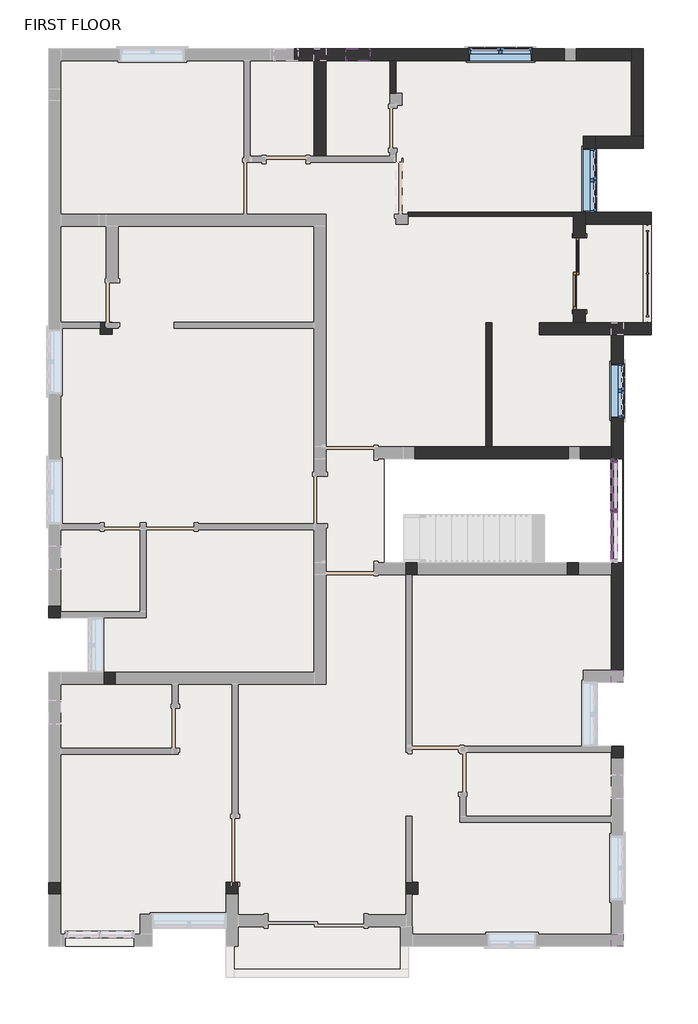
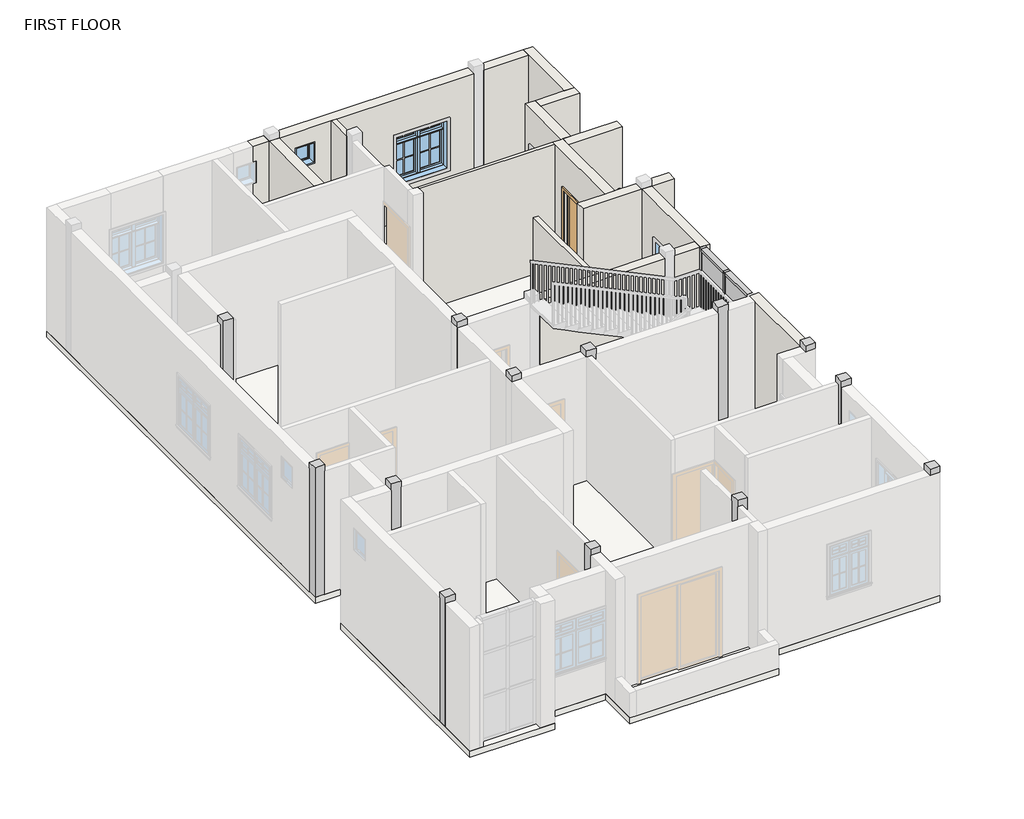
# One storey, part 3 of 6: 17 walls, 13 columns, 9 members, 4 plates, 4 windows, 1 door, 1 slab.
"""IFC4 building model written with IfcOpenShell, lengths in millimetres."""

from ifc_helpers import new_model, si_unit, frame, origin, place, context, project, spatial, polyline, outline, extrude, faceted_brep, transform, mapped, element, save
from components import door_double_sliding_4_5_x7_60868813, member_f1f71bde, member_e0487b50, member_aafbdc53, member_00c01c4d, member_0131f3aa, member_ecafcbb3, system_panel_glazed_149319f3, system_panel_glazed_118543cb, window_abb441dd, window_35f3c129, window_casement_double_awning_double_4_x4_dd9041c6

model = new_model("IFC4")

# Units and contexts
model_context = context("Model", 3, world=origin())
ifc_project = project(units=[si_unit("LENGTHUNIT", "METRE", prefix="MILLI")], contexts=[model_context])

# Site, building, storey
site = spatial("IfcSite", under=ifc_project)
building = spatial("IfcBuilding", under=site)
storey = spatial("IfcBuildingStorey", under=building, Name="FIRST FLOOR", Elevation=3200.4)

# Columns
placement = place(None, origin())
element("IfcColumn", 1, ObjectType="Rectangular Column : 9\"X9\"", at=placement, inside=storey, context=model_context, shape_type="Brep", body=[
    faceted_brep([(-5558.0284021, 3851.8787587, 3200.4), (-5786.6284021, 3851.8787587, 3200.4), (-5786.6284021, 3966.1787587, 3200.4), (-5786.6284021, 4080.4787587, 3200.4), (-5558.0284021, 4080.4787587, 3200.4), (-5558.0284021, 4074.1287587, 3200.4), (-5663.5865981, 4074.1287587, 3200.4), (-5663.5865981, 3966.1787587, 3200.4), (-5558.0284021, 3966.1787587, 3200.4), (-5558.0284021, 4080.4787587, 6400.8), (-5558.0284021, 3851.8787587, 6400.8), (-5558.0284021, 3966.1787587, 6248.4), (-5558.0284021, 4080.4787587, 6248.4), (-5786.6284021, 3851.8787587, 6400.8), (-5786.6284021, 4080.4787587, 6400.8), (-5786.6284021, 4080.4787587, 6248.4), (-5663.5865981, 4080.4787587, 6248.4), (-5663.5865981, 4080.4787587, 5334.0), (-5558.0284021, 4080.4787587, 5334.0), (-5663.5865981, 3966.1787587, 6248.4), (-5663.5865981, 4074.1287587, 5334.0), (-5558.0284021, 4074.1287587, 5334.0)], [[[0, 1, 2, 3, 4, 5, 6, 7, 8]], [[9, 10, 0, 8, 11, 12]], [[1, 0, 10, 13]], [[3, 2, 1, 13, 14, 15]], [[4, 3, 15, 14, 9, 12, 16, 17, 18]], [[10, 9, 14, 13]], [[7, 19, 11, 8]], [[19, 16, 12, 11]], [[17, 20, 21, 18]], [[20, 6, 5, 21]], [[19, 7, 6, 20, 17, 16]], [[5, 4, 18, 21]]]),
])
element("IfcColumn", 2, ObjectType="Rectangular Column : 9\"X9\"", at=placement, inside=storey, context=model_context, shape_type="Brep", body=[
    faceted_brep([(-5488.7582398, -2599.7212413, 3200.4), (-5488.7582398, -2828.3212413, 3200.4), (-5717.3582398, -2828.3212413, 3200.4), (-5717.3582398, -2599.7212413, 3200.4), (-5488.7582398, -2599.7212413, 6400.8), (-5488.7582398, -2828.3212413, 6400.8), (-5488.7582398, -2828.3212413, 6248.4), (-5488.7582398, -2599.7212413, 6248.4), (-5717.3582398, -2828.3212413, 6400.8), (-5717.3582398, -2828.3212413, 6248.4), (-5717.3582398, -2599.7212413, 6400.8), (-5717.3582398, -2599.7212413, 6248.4)], [[[0, 1, 2, 3]], [[4, 5, 6, 1, 0, 7]], [[5, 8, 9, 2, 1, 6]], [[8, 10, 11, 3, 2, 9]], [[10, 4, 7, 0, 3, 11]], [[4, 10, 8, 5]]]),
])
element("IfcColumn", 3, ObjectType="Rectangular Column : 9\"X9\"", at=placement, inside=storey, context=model_context, shape_type="Brep", body=[
    faceted_brep([(-6539.8865981, -6601.1424416, 3200.4), (-6539.8865981, -6829.7424416, 3200.4), (-6768.4865981, -6829.7424416, 3200.4), (-6768.4865981, -6601.1424416, 3200.4), (-6539.8865981, -6601.1424416, 6400.8), (-6539.8865981, -6829.7424416, 6400.8), (-6539.8865981, -6829.7424416, 6248.4), (-6539.8865981, -6601.1424416, 6248.4), (-6768.4865981, -6829.7424416, 6400.8), (-6768.4865981, -6829.7424416, 6248.4), (-6768.4865981, -6601.1424416, 6400.8), (-6768.4865981, -6601.1424416, 6248.4)], [[[0, 1, 2, 3]], [[4, 5, 6, 1, 0, 7]], [[5, 8, 9, 2, 1, 6]], [[8, 10, 11, 3, 2, 9]], [[10, 4, 7, 0, 3, 11]], [[4, 10, 8, 5]]]),
])
element("IfcColumn", 4, ObjectType="Rectangular Column : 9\"X9\"", at=placement, inside=storey, context=model_context, shape_type="Brep", body=[
    faceted_brep([(-3148.9865981, -6600.2212413, 3200.4), (-3148.9865981, -6828.8212413, 3200.4), (-3377.5865981, -6828.8212413, 3200.4), (-3377.5865981, -6600.2212413, 3200.4), (-3148.9865981, -6600.2212413, 6400.8), (-3148.9865981, -6828.8212413, 6400.8), (-3148.9865981, -6828.8212413, 6248.4), (-3148.9865981, -6600.2212413, 5334.0), (-3148.9865981, -6600.2212413, 6248.4), (-3377.5865981, -6828.8212413, 6400.8), (-3377.5865981, -6828.8212413, 6248.4), (-3377.5865981, -6600.2212413, 6400.8)], [[[0, 1, 2, 3]], [[4, 5, 6, 1, 0, 7, 8]], [[5, 9, 10, 2, 1, 6]], [[9, 11, 3, 2, 10]], [[11, 4, 8, 7, 0, 3]], [[4, 11, 9, 5]]]),
])
element("IfcColumn", 5, ObjectType="Rectangular Column : 9\"X9\"", at=placement, inside=storey, context=model_context, shape_type="Brep", body=[
    faceted_brep([(280.0134019, -6601.1424416, 3200.4), (280.0134019, -6829.7424416, 3200.4), (165.7134019, -6829.7424416, 3200.4), (51.4134019, -6829.7424416, 3200.4), (51.4134019, -6601.1424416, 3200.4), (165.7134019, -6601.1424416, 3200.4), (280.0134019, -6601.1424416, 6400.8), (280.0134019, -6829.7424416, 6400.8), (51.4134019, -6829.7424416, 6400.8), (51.4134019, -6829.7424416, 6248.4), (51.4134019, -6601.1424416, 6400.8), (51.4134019, -6601.1424416, 6248.4)], [[[0, 1, 2, 3, 4, 5]], [[6, 7, 1, 0]], [[7, 8, 9, 3, 2, 1]], [[8, 10, 11, 4, 3, 9]], [[10, 6, 0, 5, 4, 11]], [[6, 10, 8, 7]]]),
])
element("IfcColumn", 6, ObjectType="Rectangular Column : 9\"X9\"", at=placement, inside=storey, context=model_context, shape_type="SweptSolid", body=[
    extrude(outline(polyline([(4204.3134019, -7590.8212413), (4204.3134019, -7819.4212413), (3975.7134019, -7819.4212413), (3975.7134019, -7590.8212413), (4204.3134019, -7590.8212413)])), frame((0.0, 0.0, 6248.4), z_axis=(0.0, 0.0, 1.0), x_axis=(1.0, 0.0, 0.0)), (0.0, 0.0, 1.0), 152.4),
])
element("IfcColumn", 7, ObjectType="Rectangular Column : 9\"X9\"", at=placement, inside=storey, context=model_context, shape_type="Brep", body=[
    faceted_brep([(4204.3134019, -4009.4212413, 3200.4), (4204.3134019, -4238.0212413, 3200.4), (3975.7134019, -4238.0212413, 3200.4), (3975.7134019, -4123.7212413, 3200.4), (3975.7134019, -4009.4212413, 3200.4), (4204.3134019, -4009.4212413, 6400.8), (4204.3134019, -4238.0212413, 6400.8), (4204.3134019, -4238.0212413, 6248.4), (3975.7134019, -4238.0212413, 6400.8), (3975.7134019, -4238.0212413, 6248.4), (3975.7134019, -4009.4212413, 6400.8), (3975.7134019, -4009.4212413, 6248.4)], [[[0, 1, 2, 3, 4]], [[5, 6, 7, 1, 0]], [[6, 8, 9, 2, 1, 7]], [[8, 10, 11, 4, 3, 2, 9]], [[10, 5, 0, 4, 11]], [[5, 10, 8, 6]]]),
])
element("IfcColumn", 8, ObjectType="Rectangular Column : 9\"X9\"", at=placement, inside=storey, context=model_context, shape_type="Brep", body=[
    faceted_brep([(3352.7127672, -504.2212413, 3200.4), (3352.7127672, -732.8212413, 3200.4), (3124.1127672, -732.8212413, 3200.4), (3124.1127672, -504.2212413, 3200.4), (3352.7127672, -504.2212413, 6400.8), (3352.7127672, -732.8212413, 6400.8), (3352.7127672, -732.8212413, 6248.4), (3352.7127672, -504.2212413, 6248.4), (3124.1127672, -732.8212413, 6400.8), (3124.1127672, -732.8212413, 6248.4), (3124.1127672, -504.2212413, 6400.8), (3124.1127672, -504.2212413, 6248.4)], [[[0, 1, 2, 3]], [[4, 5, 6, 1, 0, 7]], [[5, 8, 9, 2, 1, 6]], [[8, 10, 11, 3, 2, 9]], [[10, 4, 7, 0, 3, 11]], [[4, 10, 8, 5]]]),
])
element("IfcColumn", 9, ObjectType="Rectangular Column : 9\"X9\"", at=placement, inside=storey, context=model_context, shape_type="Brep", body=[
    faceted_brep([(269.7035962, -504.2212413, 3200.4), (269.7035962, -732.8212413, 3200.4), (165.7134019, -732.8212413, 3200.4), (51.4134019, -732.8212413, 3200.4), (41.1035962, -732.8212413, 3200.4), (41.1035962, -504.2212413, 3200.4), (269.7035962, -504.2212413, 6400.8), (269.7035962, -732.8212413, 6400.8), (269.7035962, -732.8212413, 6248.4), (269.7035962, -504.2212413, 6248.4), (41.1035962, -732.8212413, 6400.8), (41.1035962, -732.8212413, 6248.4), (41.1035962, -504.2212413, 6400.8), (41.1035962, -504.2212413, 6248.4)], [[[0, 1, 2, 3, 4, 5]], [[6, 7, 8, 1, 0, 9]], [[7, 10, 11, 4, 3, 2, 1, 8]], [[10, 12, 13, 5, 4, 11]], [[12, 6, 9, 0, 5, 13]], [[6, 12, 10, 7]]]),
])
element("IfcColumn", 10, ObjectType="Rectangular Column : 9\"X9\"", at=placement, inside=storey, context=model_context, shape_type="Brep", body=[
    faceted_brep([(-1472.5865981, -733.7424416, 3200.4), (-1701.1865981, -733.7424416, 3200.4), (-1701.1865981, -732.8212413, 3200.4), (-1472.5865981, -732.8212413, 3200.4), (-1472.5865981, -505.1424416, 6400.8), (-1472.5865981, -733.7424416, 6400.8), (-1472.5865981, -733.7424416, 6248.4), (-1472.5865981, -732.8212413, 5334.0), (-1472.5865981, -732.8212413, 6248.4), (-1472.5865981, -505.1424416, 6248.4), (-1701.1865981, -733.7424416, 6400.8), (-1701.1865981, -733.7424416, 6248.4), (-1701.1865981, -505.1424416, 6400.8), (-1701.1865981, -505.1424416, 6248.4), (-1701.1865981, -732.8212413, 6248.4)], [[[0, 1, 2, 3]], [[4, 5, 6, 0, 3, 7, 8, 9]], [[1, 0, 6, 5, 10, 11]], [[1, 11, 10, 12, 13, 14, 2]], [[12, 4, 9, 13]], [[5, 4, 12, 10]], [[14, 8, 7, 3, 2]], [[8, 14, 13, 9]]]),
])
element("IfcColumn", 11, ObjectType="Rectangular Column : 9\"X9\"", at=placement, inside=storey, context=model_context, shape_type="Brep", body=[
    faceted_brep([(-1472.5865981, 1464.4966521, 3200.4), (-1701.1865981, 1464.4966521, 3200.4), (-1701.1865981, 1476.9787587, 3200.4), (-1472.5865981, 1476.9787587, 3200.4), (-1472.5865981, 1693.0966521, 6400.8), (-1472.5865981, 1464.4966521, 6400.8), (-1472.5865981, 1464.4966521, 6248.4), (-1472.5865981, 1476.9787587, 5334.0), (-1472.5865981, 1476.9787587, 6248.4), (-1472.5865981, 1693.0966521, 6248.4), (-1701.1865981, 1464.4966521, 6400.8), (-1701.1865981, 1464.4966521, 6248.4), (-1701.1865981, 1693.0966521, 6400.8), (-1701.1865981, 1693.0966521, 6248.4), (-1701.1865981, 1476.9787587, 6248.4)], [[[0, 1, 2, 3]], [[4, 5, 6, 0, 3, 7, 8, 9]], [[1, 0, 6, 5, 10, 11]], [[1, 11, 10, 12, 13, 14, 2]], [[12, 4, 9, 13]], [[5, 4, 12, 10]], [[14, 8, 7, 3, 2]], [[8, 14, 13, 9]]]),
])
element("IfcColumn", 12, ObjectType="Rectangular Column : 9\"X9\"", at=placement, inside=storey, context=model_context, shape_type="Brep", body=[
    faceted_brep([(-6539.8865981, -1329.7212413, 3200.4), (-6539.8865981, -1444.0212413, 3200.4), (-6539.8865981, -1558.3212413, 3200.4), (-6768.4865981, -1558.3212413, 3200.4), (-6768.4865981, -1329.7212413, 3200.4), (-6539.8865981, -1329.7212413, 6400.8), (-6539.8865981, -1558.3212413, 6400.8), (-6539.8865981, -1558.3212413, 6248.4), (-6539.8865981, -1329.7212413, 6248.4), (-6768.4865981, -1558.3212413, 6400.8), (-6768.4865981, -1329.7212413, 6400.8), (-6768.4865981, -1329.7212413, 6248.4)], [[[0, 1, 2, 3, 4]], [[5, 6, 7, 2, 1, 0, 8]], [[6, 9, 3, 2, 7]], [[9, 10, 11, 4, 3]], [[10, 5, 8, 0, 4, 11]], [[5, 10, 9, 6]]]),
])
element("IfcColumn", 13, ObjectType="Rectangular Column : 9\"X9\"", at=placement, inside=storey, context=model_context, shape_type="SweptSolid", body=[
    extrude(outline(polyline([(4204.3134019, -2561.6212413), (4204.3134019, -2790.2212413), (3975.7134019, -2790.2212413), (3975.7134019, -2561.6212413), (4204.3134019, -2561.6212413)])), frame((0.0, 0.0, 6248.4), z_axis=(0.0, 0.0, 1.0), x_axis=(1.0, 0.0, 0.0)), (0.0, 0.0, 1.0), 152.4),
])

# Door
door_double_sliding_4_5_x7_shape = door_double_sliding_4_5_x7_60868813(model_context)
element("IfcDoor", 14, ObjectType="Door-Double-Sliding : 4.5'X7'", at=placement, inside=storey, context=model_context, shape_type="MappedRepresentation", body=[
    mapped(door_double_sliding_4_5_x7_shape, transform((3493.1134019, 5007.5787587, 3200.4), x_axis=(0.0, 1.0, 0.0), y_axis=(-1.0, 0.0, 0.0), z_axis=(0.0, 0.0, 1.0))),
])

# Members
member_shape = member_f1f71bde(model_context)
element("IfcMember", 15, ObjectType="Rectangular Mullion : 2.5\" x 5\" rectangular", at=placement, inside=storey, context=model_context, shape_type="MappedRepresentation", body=[
    mapped(member_shape, transform((4026.5134019, 1413.4787587, 6248.4), x_axis=(0.0, 0.0, 1.0), y_axis=(1.0, 0.0, 0.0), z_axis=(0.0, 1.0, 0.0))),
])
element("IfcMember", 16, ObjectType="Rectangular Mullion : 2.5\" x 5\" rectangular", at=placement, inside=storey, context=model_context, shape_type="MappedRepresentation", body=[
    mapped(member_shape, transform((4026.5134019, 454.6287587, 6248.4), x_axis=(0.0, 0.0, 1.0), y_axis=(1.0, 0.0, 0.0), z_axis=(0.0, 1.0, 0.0))),
])
element("IfcMember", 17, ObjectType="Rectangular Mullion : 2.5\" x 5\" rectangular", at=placement, inside=storey, context=model_context, shape_type="MappedRepresentation", body=[
    mapped(member_shape, transform((4026.5134019, 518.1287587, 3200.4), x_axis=(0.0, 0.0, -1.0), y_axis=(1.0, 0.0, 0.0), z_axis=(0.0, -1.0, 0.0))),
])
member_2_shape = member_e0487b50(model_context)
element("IfcMember", 18, ObjectType="Rectangular Mullion : 2.5\" x 5\" rectangular", at=placement, inside=storey, context=model_context, shape_type="MappedRepresentation", body=[
    mapped(member_2_shape, transform((4026.5134019, 454.6287587, 4756.15), x_axis=(0.0, 0.0, 1.0), y_axis=(1.0, 0.0, 0.0), z_axis=(0.0, 1.0, 0.0))),
])
element("IfcMember", 19, ObjectType="Rectangular Mullion : 2.5\" x 5\" rectangular", at=placement, inside=storey, context=model_context, shape_type="MappedRepresentation", body=[
    mapped(member_2_shape, transform((4026.5134019, 1413.4787587, 4756.15), x_axis=(0.0, 0.0, 1.0), y_axis=(1.0, 0.0, 0.0), z_axis=(0.0, 1.0, 0.0))),
])
member_3_shape = member_aafbdc53(model_context)
element("IfcMember", 20, ObjectType="Rectangular Mullion : 2.5\" x 5\" rectangular", at=placement, inside=storey, context=model_context, shape_type="MappedRepresentation", body=[
    mapped(member_3_shape, transform((4026.5134019, 486.3787587, 3200.4), x_axis=(0.0, 1.0, 0.0), y_axis=(1.0, 0.0, 0.0), z_axis=(0.0, 0.0, -1.0))),
])
member_4_shape = member_00c01c4d(model_context)
element("IfcMember", 21, ObjectType="Rectangular Mullion : 2.5\" x 5\" rectangular", at=placement, inside=storey, context=model_context, shape_type="MappedRepresentation", body=[
    mapped(member_4_shape, transform((4026.5134019, 1476.9787587, 3200.4), x_axis=(0.0, 1.0, 0.0), y_axis=(1.0, 0.0, 0.0), z_axis=(0.0, 0.0, -1.0))),
])
member_5_shape = member_0131f3aa(model_context)
element("IfcMember", 22, ObjectType="Rectangular Mullion : 2.5\" x 5\" rectangular", at=placement, inside=storey, context=model_context, shape_type="MappedRepresentation", body=[
    mapped(member_5_shape, transform((4026.5134019, 486.3787587, 4756.15), x_axis=(0.0, 1.0, 0.0), y_axis=(1.0, 0.0, 0.0), z_axis=(0.0, 0.0, -1.0))),
])
member_6_shape = member_ecafcbb3(model_context)
element("IfcMember", 23, ObjectType="Rectangular Mullion : 2.5\" x 5\" rectangular", at=placement, inside=storey, context=model_context, shape_type="MappedRepresentation", body=[
    mapped(member_6_shape, transform((4026.5134019, 1476.9787587, 4756.15), x_axis=(0.0, 1.0, 0.0), y_axis=(1.0, 0.0, 0.0), z_axis=(0.0, 0.0, -1.0))),
])

# Plates
system_panel_glazed_shape = system_panel_glazed_149319f3(model_context)
element("IfcPlate", 24, ObjectType="System Panel : Glazed", at=placement, inside=storey, context=model_context, shape_type="MappedRepresentation", body=[
    mapped(system_panel_glazed_shape, transform((4026.5134019, 6.9537587, 3263.9), x_axis=(0.0, 1.0, 0.0), y_axis=(-1.0, 0.0, 0.0), z_axis=(0.0, 0.0, 1.0))),
])
element("IfcPlate", 25, ObjectType="System Panel : Glazed", at=placement, inside=storey, context=model_context, shape_type="MappedRepresentation", body=[
    mapped(system_panel_glazed_shape, transform((4026.5134019, 965.8037587, 3263.9), x_axis=(0.0, 1.0, 0.0), y_axis=(-1.0, 0.0, 0.0), z_axis=(0.0, 0.0, 1.0))),
])
system_panel_glazed_2_shape = system_panel_glazed_118543cb(model_context)
element("IfcPlate", 26, ObjectType="System Panel : Glazed", at=placement, inside=storey, context=model_context, shape_type="MappedRepresentation", body=[
    mapped(system_panel_glazed_2_shape, transform((4026.5134019, 6.9537587, 4787.9), x_axis=(0.0, 1.0, 0.0), y_axis=(-1.0, 0.0, 0.0), z_axis=(0.0, 0.0, 1.0))),
])
element("IfcPlate", 27, ObjectType="System Panel : Glazed", at=placement, inside=storey, context=model_context, shape_type="MappedRepresentation", body=[
    mapped(system_panel_glazed_2_shape, transform((4026.5134019, 965.8037587, 4787.9), x_axis=(0.0, 1.0, 0.0), y_axis=(-1.0, 0.0, 0.0), z_axis=(0.0, 0.0, 1.0))),
])

# Slab
element("IfcSlab", 28, ObjectType="6\"", at=placement, inside=storey, context=model_context, shape_type="SweptSolid", body=[
    extrude(outline(polyline([(-6768.4865981, -1558.3212413), (-6768.4865981, 9300.1787587), (4585.3134019, 9300.1787587), (4585.3134019, 7395.1787587), (3670.9134019, 7395.1787587), (3670.9134019, 6175.9787587), (4737.7134019, 6175.9787587), (4737.7134019, 3839.1787587), (4204.3134019, 3839.1787587), (4204.3134019, -2790.2212413), (3670.9134019, -2790.2212413), (3670.9134019, -4009.4212413), (4204.3134019, -4009.4212413), (4204.3134019, -7819.4212413), (102.2134019, -7819.4212413), (102.2134019, -8416.3212413), (-3377.5865981, -8416.3212413), (-3377.5865981, -7438.4212413), (-4787.2865981, -7438.4212413), (-4787.2865981, -7819.4212413), (-6768.4865981, -7819.4212413), (-6768.4865981, -2599.7212413), (-5974.2886947, -2599.7212413), (-5974.2886947, -1558.3212413), (-6768.4865981, -1558.3212413)]), holes=[polyline([(4178.9134019, 1705.5787587), (-353.2951421, 1705.5787587), (-353.2951421, -732.8212413), (4178.9134019, -732.8212413), (4178.9134019, 1705.5787587)])]), frame((0.0, 0.0, 3048.0), z_axis=(0.0, 0.0, 1.0), x_axis=(1.0, 0.0, 0.0)), (0.0, 0.0, 1.0), 152.4),
])

# Walls
element("IfcWall", 29, ObjectType="3\"", at=placement, inside=storey, context=model_context, shape_type="Brep", body=[
    faceted_brep([(3251.8134019, 6175.9787587, 3200.4), (89.5134019, 6175.9787587, 3200.4), (89.5134019, 6175.9787587, 5334.0), (89.5134019, 6175.9787587, 6248.4), (3251.8134019, 6175.9787587, 6248.4), (3251.8134019, 6099.7787587, 3200.4), (3251.8134019, 6099.7787587, 6248.4), (89.5134019, 6099.7787587, 6248.4), (89.5134019, 6099.7787587, 3200.4), (89.5134019, 6137.8787587, 3200.4)], [[[0, 1, 2, 3, 4]], [[5, 6, 7, 8]], [[1, 0, 5, 8, 9]], [[4, 3, 7, 6]], [[0, 4, 6, 5]], [[3, 2, 1, 9, 8, 7]]]),
])
element("IfcWall", 30, ObjectType="4.5\"", at=placement, inside=storey, context=model_context, shape_type="SweptSolid", body=[
    extrude(outline(polyline([(-139.0865981, 9071.5787587), (-139.0865981, 8443.0921256), (-253.3865981, 8443.0921256), (-253.3865981, 9071.5787587), (-139.0865981, 9071.5787587)])), frame((0.0, 0.0, 3200.4), z_axis=(0.0, 0.0, 1.0), x_axis=(1.0, 0.0, 0.0)), (0.0, 0.0, 1.0), 3048.0),
])
element("IfcWall", 31, ObjectType="4.5\"", at=placement, inside=storey, context=model_context, shape_type="SweptSolid", body=[
    extrude(outline(polyline([(1575.4134019, 1705.5787587), (1575.4134019, 4067.7787587), (1689.7134019, 4067.7787587), (1689.7134019, 1705.5787587), (1575.4134019, 1705.5787587)])), frame((0.0, 0.0, 3200.4), z_axis=(0.0, 0.0, 1.0), x_axis=(1.0, 0.0, 0.0)), (0.0, 0.0, 1.0), 3048.0),
])
element("IfcWall", 32, ObjectType="6\"", at=placement, inside=storey, context=model_context, shape_type="SweptSolid", body=[
    extrude(outline(polyline([(4585.3134019, 4067.7787587), (4585.3134019, 5947.3787587), (4737.7134019, 5947.3787587), (4737.7134019, 4067.7787587), (4585.3134019, 4067.7787587)])), frame((0.0, 0.0, 3200.4), z_axis=(0.0, 0.0, 1.0), x_axis=(1.0, 0.0, 0.0)), (0.0, 0.0, 1.0), 609.6),
])
element("IfcWall", 33, ObjectType="9\"", at=placement, inside=storey, context=model_context, shape_type="Brep", body=[
    faceted_brep([(4204.3134019, -2561.6212413, 6248.4), (4204.3134019, -2561.6212413, 3200.4), (4204.3134019, -504.2212413, 3200.4), (4204.3134019, -504.2212413, 6248.4), (3975.7134019, -2561.6212413, 3200.4), (3975.7134019, -2561.6212413, 6248.4), (3975.7134019, -732.8212413, 6248.4), (3975.7134019, -504.2212413, 6248.4), (3975.7134019, -504.2212413, 3200.4), (3975.7134019, -732.8212413, 3200.4)], [[[0, 1, 2, 3]], [[4, 5, 6, 7, 8, 9]], [[1, 4, 9, 8, 2]], [[5, 0, 3, 7, 6]], [[1, 0, 5, 4]], [[3, 2, 8, 7]]]),
    faceted_brep([(4204.3134019, 3839.1787587, 3200.4), (4204.3134019, 3839.1787587, 6248.4), (4204.3134019, 1476.9787587, 6248.4), (4204.3134019, 1476.9787587, 3200.4), (4204.3134019, 2251.6787587, 5334.0), (4204.3134019, 3293.0787587, 5334.0), (4204.3134019, 3293.0787587, 4114.8), (4204.3134019, 2251.6787587, 4114.8), (3975.7134019, 3839.1787587, 6248.4), (3975.7134019, 3839.1787587, 3200.4), (3975.7134019, 1705.5787587, 3200.4), (3975.7134019, 1476.9787587, 3200.4), (3975.7134019, 1476.9787587, 6248.4), (3975.7134019, 1705.5787587, 6248.4), (3975.7134019, 2251.6787587, 5334.0), (3975.7134019, 2251.6787587, 4114.8), (3975.7134019, 3293.0787587, 4114.8), (3975.7134019, 3293.0787587, 5334.0)], [[[0, 1, 2, 3], [4, 5, 6, 7]], [[8, 9, 10, 11, 12, 13], [14, 15, 16, 17]], [[9, 0, 3, 11, 10]], [[1, 8, 13, 12, 2]], [[1, 0, 9, 8]], [[15, 14, 4, 7]], [[16, 15, 7, 6]], [[17, 16, 6, 5]], [[14, 17, 5, 4]], [[3, 2, 12, 11]]]),
])
element("IfcWall", 34, ObjectType="9\"", at=placement, inside=storey, context=model_context, shape_type="Brep", body=[
    faceted_brep([(229.251657, 1476.9787587, 3200.4), (3156.5070369, 1476.9787587, 3200.4), (3156.5070369, 1476.9787587, 6248.4), (229.251657, 1476.9787587, 6248.4), (229.251657, 1705.5787587, 3200.4), (229.251657, 1705.5787587, 6248.4), (1575.4134019, 1705.5787587, 6248.4), (1689.7134019, 1705.5787587, 6248.4), (3156.5070369, 1705.5787587, 6248.4), (3156.5070369, 1705.5787587, 3200.4), (1689.7134019, 1705.5787587, 3200.4), (1575.4134019, 1705.5787587, 3200.4)], [[[0, 1, 2, 3]], [[4, 5, 6, 7, 8, 9, 10, 11]], [[1, 0, 4, 11, 10, 9]], [[2, 1, 9, 8]], [[3, 2, 8, 7, 6, 5]], [[0, 3, 5, 4]]]),
])
element("IfcWall", 35, ObjectType="9\"", at=placement, inside=storey, context=model_context, shape_type="SweptSolid", body=[
    extrude(outline(polyline([(3975.7134019, 1476.9787587), (3385.1070369, 1476.9787587), (3385.1070369, 1705.5787587), (3975.7134019, 1705.5787587), (3975.7134019, 1476.9787587)])), frame((0.0, 0.0, 3200.4), z_axis=(0.0, 0.0, 1.0), x_axis=(1.0, 0.0, 0.0)), (0.0, 0.0, 1.0), 3048.0),
])
element("IfcWall", 36, ObjectType="9\"", at=placement, inside=storey, context=model_context, shape_type="Brep", body=[
    faceted_brep([(2604.1134019, 3839.1787587, 3200.4), (3975.7134019, 3839.1787587, 3200.4), (4204.3134019, 3839.1787587, 3200.4), (4737.7134019, 3839.1787587, 3200.4), (4737.7134019, 3839.1787587, 6248.4), (4204.3134019, 3839.1787587, 6248.4), (3975.7134019, 3839.1787587, 6248.4), (2604.1134019, 3839.1787587, 6248.4), (2604.1134019, 4067.7787587, 3200.4), (2604.1134019, 4067.7787587, 6248.4), (3251.8134019, 4067.7787587, 6248.4), (3480.4134019, 4067.7787587, 6248.4), (3975.7134019, 4067.7787587, 6248.4), (4204.3134019, 4067.7787587, 6248.4), (4737.7134019, 4067.7787587, 6248.4), (4737.7134019, 4067.7787587, 3810.0), (4737.7134019, 4067.7787587, 3200.4), (4585.3134019, 4067.7787587, 3200.4), (3480.4134019, 4067.7787587, 3200.4), (3251.8134019, 4067.7787587, 3200.4)], [[[0, 1, 2, 3, 4, 5, 6, 7]], [[8, 9, 10, 11, 12, 13, 14, 15, 16, 17, 18, 19]], [[3, 2, 1, 0, 8, 19, 18, 17, 16]], [[7, 6, 5, 4, 14, 13, 12, 11, 10, 9]], [[0, 7, 9, 8]], [[4, 3, 16, 15, 14]]]),
])
element("IfcWall", 37, ObjectType="9\"", at=placement, inside=storey, context=model_context, shape_type="Brep", body=[
    faceted_brep([(3480.4134019, 5693.3787587, 5334.0), (3480.4134019, 5693.3787587, 3200.4), (3480.4134019, 5947.3787587, 3200.4), (3480.4134019, 6175.9787587, 3200.4), (3480.4134019, 6175.9787587, 6248.4), (3480.4134019, 5947.3787587, 6248.4), (3480.4134019, 4067.7787587, 6248.4), (3480.4134019, 4067.7787587, 3200.4), (3480.4134019, 4321.7787587, 3200.4), (3480.4134019, 4321.7787587, 5334.0), (3251.8134019, 6175.9787587, 3200.4), (3251.8134019, 6099.7787587, 3200.4), (3251.8134019, 5693.3787587, 3200.4), (3251.8134019, 5693.3787587, 5334.0), (3251.8134019, 4321.7787587, 5334.0), (3251.8134019, 4321.7787587, 3200.4), (3251.8134019, 4067.7787587, 3200.4), (3251.8134019, 4067.7787587, 6248.4), (3251.8134019, 6099.7787587, 6248.4), (3251.8134019, 6175.9787587, 6248.4), (3442.3134019, 6175.9787587, 3200.4), (3442.3134019, 6175.9787587, 6248.4)], [[[0, 1, 2, 3, 4, 5, 6, 7, 8, 9]], [[10, 11, 12, 13, 14, 15, 16, 17, 18, 19]], [[8, 7, 16, 15]], [[3, 2, 1, 12, 11, 10, 20]], [[6, 5, 4, 21, 19, 18, 17]], [[7, 6, 17, 16]], [[4, 3, 20, 10, 19, 21]], [[15, 14, 9, 8]], [[13, 12, 1, 0]], [[14, 13, 0, 9]]]),
])
element("IfcWall", 38, ObjectType="9\"", at=placement, inside=storey, context=model_context, shape_type="Brep", body=[
    faceted_brep([(3480.4134019, 5947.3787587, 3200.4), (4585.3134019, 5947.3787587, 3200.4), (4737.7134019, 5947.3787587, 3200.4), (4737.7134019, 5947.3787587, 3810.0), (4737.7134019, 5947.3787587, 6248.4), (3480.4134019, 5947.3787587, 6248.4), (3480.4134019, 6175.9787587, 3200.4), (3480.4134019, 6175.9787587, 6248.4), (3670.9134019, 6175.9787587, 6248.4), (4737.7134019, 6175.9787587, 6248.4), (4737.7134019, 6175.9787587, 3200.4), (3670.9134019, 6175.9787587, 3200.4)], [[[0, 1, 2, 3, 4, 5]], [[6, 7, 8, 9, 10, 11]], [[2, 1, 0, 6, 11, 10]], [[5, 4, 9, 8, 7]], [[0, 5, 7, 6]], [[4, 3, 2, 10, 9]]]),
])
element("IfcWall", 39, ObjectType="9\"", at=placement, inside=storey, context=model_context, shape_type="Brep", body=[
    faceted_brep([(3670.9134019, 7395.1787587, 4114.8), (3670.9134019, 6175.9787587, 4114.8), (3670.9134019, 6175.9787587, 3200.4), (3670.9134019, 7395.1787587, 3200.4), (3670.9134019, 7623.7787587, 3200.4), (3670.9134019, 7623.7787587, 6248.4), (3670.9134019, 7395.1787587, 6248.4), (3670.9134019, 6175.9787587, 6248.4), (3670.9134019, 6175.9787587, 5334.0), (3670.9134019, 7395.1787587, 5334.0), (3442.3134019, 6175.9787587, 3200.4), (3442.3134019, 6175.9787587, 4114.8), (3442.3134019, 7395.1787587, 4114.8), (3442.3134019, 7395.1787587, 5334.0), (3442.3134019, 6175.9787587, 5334.0), (3442.3134019, 6175.9787587, 6248.4), (3442.3134019, 7623.7787587, 6248.4), (3442.3134019, 7623.7787587, 3200.4), (3480.4134019, 6175.9787587, 3200.4), (3480.4134019, 6175.9787587, 6248.4)], [[[0, 1, 2, 3, 4, 5, 6, 7, 8, 9]], [[10, 11, 12, 13, 14, 15, 16, 17]], [[4, 3, 2, 18, 10, 17]], [[7, 6, 5, 16, 15, 19]], [[8, 7, 19, 15, 14]], [[2, 1, 11, 10, 18]], [[5, 4, 17, 16]], [[12, 11, 1, 0]], [[13, 12, 0, 9]], [[14, 13, 9, 8]]]),
])
element("IfcWall", 40, ObjectType="9\"", at=placement, inside=storey, context=model_context, shape_type="Brep", body=[
    faceted_brep([(3670.9134019, 7395.1787587, 3200.4), (4585.3134019, 7395.1787587, 3200.4), (4585.3134019, 7395.1787587, 6248.4), (3670.9134019, 7395.1787587, 6248.4), (3670.9134019, 7395.1787587, 5334.0), (3670.9134019, 7395.1787587, 4114.8), (3670.9134019, 7623.7787587, 3200.4), (3670.9134019, 7623.7787587, 6248.4), (4356.7134019, 7623.7787587, 6248.4), (4585.3134019, 7623.7787587, 6248.4), (4585.3134019, 7623.7787587, 3200.4), (4356.7134019, 7623.7787587, 3200.4)], [[[0, 1, 2, 3, 4, 5]], [[6, 7, 8, 9, 10, 11]], [[1, 0, 6, 11, 10]], [[3, 2, 9, 8, 7]], [[0, 5, 4, 3, 7, 6]], [[2, 1, 10, 9]]]),
])
element("IfcWall", 41, ObjectType="9\"", at=placement, inside=storey, context=model_context, shape_type="Brep", body=[
    faceted_brep([(4585.3134019, 7623.7787587, 3200.4), (4585.3134019, 9300.1787587, 3200.4), (4585.3134019, 9300.1787587, 6248.4), (4585.3134019, 7623.7787587, 6248.4), (4356.7134019, 7623.7787587, 3200.4), (4356.7134019, 7623.7787587, 6248.4), (4356.7134019, 9071.5787587, 6248.4), (4356.7134019, 9300.1787587, 6248.4), (4356.7134019, 9300.1787587, 3200.4), (4356.7134019, 9071.5787587, 3200.4)], [[[0, 1, 2, 3]], [[4, 5, 6, 7, 8, 9]], [[1, 0, 4, 9, 8]], [[3, 2, 7, 6, 5]], [[0, 3, 5, 4]], [[2, 1, 8, 7]]]),
])
element("IfcWall", 42, ObjectType="9\"", at=placement, inside=storey, context=model_context, shape_type="SweptSolid", body=[
    extrude(outline(polyline([(3305.8577655, 9300.1787587), (4356.7134019, 9300.1787587), (4356.7134019, 9071.5787587), (3305.8577655, 9071.5787587), (3305.8577655, 9300.1787587)])), frame((0.0, 0.0, 3200.4), z_axis=(0.0, 0.0, 1.0), x_axis=(1.0, 0.0, 0.0)), (0.0, 0.0, 1.0), 3048.0),
])
element("IfcWall", 43, ObjectType="9\"", at=placement, inside=storey, context=model_context, shape_type="Brep", body=[
    faceted_brep([(3077.2577655, 9300.1787587, 3200.4), (-1701.1865981, 9300.1787587, 3200.4), (-1701.1865981, 9300.1787587, 6248.4), (-1472.5865981, 9300.1787587, 6248.4), (3077.2577655, 9300.1787587, 6248.4), (-634.3865981, 9300.1787587, 5867.4), (-1091.5865981, 9300.1787587, 5867.4), (-1091.5865981, 9300.1787587, 5334.0), (-634.3865981, 9300.1787587, 5334.0), (2467.6577655, 9300.1787587, 5334.0), (1248.4577655, 9300.1787587, 5334.0), (1248.4577655, 9300.1787587, 4114.8), (2467.6577655, 9300.1787587, 4114.8), (3077.2577655, 9071.5787587, 3200.4), (3077.2577655, 9071.5787587, 6248.4), (-139.0865981, 9071.5787587, 6248.4), (-253.3865981, 9071.5787587, 6248.4), (-1472.5865981, 9071.5787587, 6248.4), (-1701.1865981, 9071.5787587, 6248.4), (-1701.1865981, 9071.5787587, 3200.4), (-1472.5865981, 9071.5787587, 3200.4), (-253.3865981, 9071.5787587, 3200.4), (-139.0865981, 9071.5787587, 3200.4), (-634.3865981, 9071.5787587, 5867.4), (-634.3865981, 9071.5787587, 5334.0), (-1091.5865981, 9071.5787587, 5334.0), (-1091.5865981, 9071.5787587, 5867.4), (2467.6577655, 9071.5787587, 5334.0), (2467.6577655, 9071.5787587, 4114.8), (1248.4577655, 9071.5787587, 4114.8), (1248.4577655, 9071.5787587, 5334.0)], [[[0, 1, 2, 3, 4], [5, 6, 7, 8], [9, 10, 11, 12]], [[13, 14, 15, 16, 17, 18, 19, 20, 21, 22], [23, 24, 25, 26], [27, 28, 29, 30]], [[1, 0, 13, 22, 21, 20, 19]], [[4, 3, 2, 18, 17, 16, 15, 14]], [[0, 4, 14, 13]], [[2, 1, 19, 18]], [[24, 23, 5, 8]], [[25, 24, 8, 7]], [[26, 25, 7, 6]], [[23, 26, 6, 5]], [[28, 27, 9, 12]], [[29, 28, 12, 11]], [[30, 29, 11, 10]], [[27, 30, 10, 9]]]),
])
element("IfcWall", 44, ObjectType="9\"", at=placement, inside=storey, context=model_context, shape_type="SweptSolid", body=[
    extrude(outline(polyline([(3200.4, -2082.1865981), (3200.4, -1701.1865981), (6248.4, -1701.1865981), (6248.4, -2082.1865981), (5867.4, -2082.1865981), (5867.4, -2005.9865981), (5334.0, -2005.9865981), (5334.0, -2082.1865981), (3200.4, -2082.1865981)])), frame((0.0, 9071.5787587, 0.0), z_axis=(0.0, 1.0, 0.0), x_axis=(0.0, 0.0, 1.0)), (0.0, 0.0, 1.0), 228.6),
])
element("IfcWall", 45, ObjectType="9\"", at=placement, inside=storey, context=model_context, shape_type="SweptSolid", body=[
    extrude(outline(polyline([(-1701.1865981, 7242.7787587), (-1701.1865981, 9071.5787587), (-1472.5865981, 9071.5787587), (-1472.5865981, 7242.7787587), (-1701.1865981, 7242.7787587)])), frame((0.0, 0.0, 3200.4), z_axis=(0.0, 0.0, 1.0), x_axis=(1.0, 0.0, 0.0)), (0.0, 0.0, 1.0), 3048.0),
])

# Windows
window_shape = window_abb441dd(model_context)
element("IfcWindow", 46, ObjectType="Fixed : 1'6\"X1'9\"", at=placement, inside=storey, context=model_context, shape_type="MappedRepresentation", body=[
    mapped(window_shape, transform((-824.8865981, 9185.8787587, 3200.4), x_axis=(1.0, 0.0, 0.0), y_axis=(0.0, 1.0, 0.0), z_axis=(0.0, 0.0, 1.0))),
])
window_2_shape = window_35f3c129(model_context)
element("IfcWindow", 47, ObjectType="Window-Casement-Double-Awning-Double : 3'5\"X7'", at=placement, inside=storey, context=model_context, shape_type="MappedRepresentation", body=[
    mapped(window_2_shape, transform((4090.0134019, 2772.3787587, 3200.4), x_axis=(0.0, -1.0, 0.0), y_axis=(1.0, 0.0, 0.0), z_axis=(0.0, 0.0, 1.0))),
])
window_casement_double_awning_double_4_x4_shape = window_casement_double_awning_double_4_x4_dd9041c6(model_context)
element("IfcWindow", 48, ObjectType="Window-Casement-Double-Awning-Double : 4'X4'", at=placement, inside=storey, context=model_context, shape_type="MappedRepresentation", body=[
    mapped(window_casement_double_awning_double_4_x4_shape, transform((3556.6134019, 6785.5787587, 3200.4), x_axis=(0.0, -1.0, 0.0), y_axis=(1.0, 0.0, 0.0), z_axis=(0.0, 0.0, 1.0))),
])
element("IfcWindow", 49, ObjectType="Window-Casement-Double-Awning-Double : 4'X4'", at=placement, inside=storey, context=model_context, shape_type="MappedRepresentation", body=[
    mapped(window_casement_double_awning_double_4_x4_shape, transform((1858.0577655, 9185.8787587, 3200.4), x_axis=(1.0, 0.0, 0.0), y_axis=(0.0, 1.0, 0.0), z_axis=(0.0, 0.0, 1.0))),
])

save(model, "model.ifc")

# Revit data of these elements
# Type "Rectangular Column : 9\"X9\""
#   Assembly Code = "B1010200"
#   Depth = 0' - 9"
#   Offset Base = 0' - 0"
#   Offset Top = 0' - 0"
#   Width = 0' - 9"
#   Material = none
# Type "Door-Double-Sliding : 4.5'X7'"
#   Type Mark = "14"
#   Construction Type Id = "opn-d45"
#   Assembly Code = "C1020"
#   Analytic Construction = "Wood frame, double glass door "
#   Thickness = 0' - 2"
#   Thermal Resistance (R) = 1.8150 (h·ft²·°F)/BTU
#   Heat Transfer Coefficient (U) = 0.5510 BTU/(h·ft²·°F)
#   Height = 7' - 0"
#   Rail Width = 0' - 2"
#   Stiles = 0' - 2"
#   Trim Projection Ext = 0' - 1"
#   Trim Projection Int = 0' - 1"
#   Trim Width = 0' - 3"
#   Width = 4' - 6"
#   Define Thermal Properties by = 1
#   Glazing = Glass
#   Panel Material = Wood - Birch - Solid Stained Light Low Gloss
#   Trim Material = Paint - Sienna
#   Visual Light Transmittance = 0
#   Solar Heat Gain Coefficient = 0
#   Function = (empty or 0)
#   Wall Closure = (empty or 0)
# Type "Rectangular Mullion : 2.5\" x 5\" rectangular"
#   built-in parameter 1007304 = 0.416667 (stored number, unit not read)
#   built-in parameter 1007301 = 0.104167 (stored number, unit not read)
#   built-in parameter 1007300 = 0.104167 (stored number, unit not read)
# Type "System Panel : Glazed"
#   Construction Type Id = "GSP4R"
#   Analytic Construction = "1/8 in Pilkington single glazing"
#   Visual Light Transmittance = 0.9
#   Solar Heat Gain Coefficient = 0.86
#   Heat Transfer Coefficient (U) = 1.18115 BTU/(h·ft²·°F)
#   Define Thermal Properties by = 1
# Type "6\""
#   Assembly Code = "B1010"
#   Function = 0
#   Layers, outside or top first: 0' - 6" no material (function 1)
# Type "3\""
#   Assembly Code = "B2010"
#   Layers, outside or top first: 0' - 3" no material (function 1)
# Type "4.5\""
#   Assembly Code = "B2010"
#   Layers, outside or top first: 0' - 4 1/2" no material (function 1)
# Type "6\""
#   Assembly Code = "B2010"
#   Layers, outside or top first: 0' - 6" "wood 1" (function 1)
# Type "9\""
#   Assembly Code = "B2010"
#   Layers, outside or top first: 0' - 9" "wall" (function 1)
# Type "Fixed : 1'6\"X1'9\""
#   Type Mark = "24"
#   Construction Type Id = "GSP4R"
#   Assembly Code = "B2020100"
#   Analytic Construction = "1/8 in Pilkington single glazing"
#   Visual Light Transmittance = 0.9
#   Solar Heat Gain Coefficient = 0.78
#   Heat Transfer Coefficient (U) = 0.6496 BTU/(h·ft²·°F)
#   Height = 1' - 9"
#   Default Sill Height = 7' - 0"
#   Width = 1' - 6"
#   Window Inset = 0' - 0 3/4"
#   Define Thermal Properties by = 1
#   Glass Pane Material = Glass
#   Sash Material = Sash
#   Wall Closure = (empty or 0)
# Type "Window-Casement-Double-Awning-Double : 3'5\"X7'"
#   Type Mark = "22"
#   Fire Rating = "0.5h"
#   Assembly Code = "B2020100"
#   Analytic Construction = "Double glazing - domestic"
#   Window Inset [instance default] = 0' - 0"
#   Wall Thickness [instance default] = 0' - 6"
#   Interior Wall Closure [instance default] = 0' - 2 1/4"
#   Half Width = 1' - 8 1/2"
#   Visual Light Transmittance = 0.81
#   Transom Height = 1' - 0"
#   Thermal Resistance (R) = 1.8146 (h·ft²·°F)/BTU
#   Solar Heat Gain Coefficient = 0.76
#   Rough Width = 3' - 5 1/2"
#   Rough Height = 4' - 0 1/2"
#   Open Window Height = 3' - 0"
#   Frame Extension [instance default] = 0' - 0 1/4"
#   Height = 4' - 0"
#   Heat Transfer Coefficient (U) = 0.5511 BTU/(h·ft²·°F)
#   Exterior Wall Closure [instance default] = 0' - 1 1/4"
#   Extension Jamb [instance default] = 0' - 2 1/4"
#   Default Sill Height = 3' - 0"
#   Width = 3' - 5"
#   Top Muntin Visibility = yes
#   Bottom Muntin Visibility = yes
#   Interior Trim Visibility [instance default] = yes
#   Exterior Trim Visibility [instance default] = yes
#   Extension Jamb Visibility [instance default] = yes
#   Interior Trim Material = Wood - Stained
#   Muntin Pattern = Muntin Pattern_2x2 : Muntin Pattern_2x2
#   Interior Trim = Trim-Window-Interior-Flat : Picture Frame
#   Interior Frame Material = Wood - Stained
#   Glass Panel Material = Glass
#   Exterior Trim Material = Clad - White
#   Exterior Trim = Trim-Window-Exterior-Flat : with Sill
#   Exterior Frame Material = Clad - White
#   Wall Closure = (empty or 0)
# Type "Window-Casement-Double-Awning-Double : 4'X4'"
#   Type Mark = "19"
#   Fire Rating = "0.5h"
#   Assembly Code = "B2020100"
#   Analytic Construction = "Double glazing - domestic"
#   Window Inset [instance default] = 0' - 0"
#   Wall Thickness [instance default] = 0' - 6"
#   Interior Wall Closure [instance default] = 0' - 2 1/4"
#   Half Width = 2' - 0"
#   Visual Light Transmittance = 0.81
#   Transom Height = 1' - 0"
#   Thermal Resistance (R) = 1.8146 (h·ft²·°F)/BTU
#   Solar Heat Gain Coefficient = 0.76
#   Rough Width = 4' - 0 1/2"
#   Rough Height = 4' - 0 1/2"
#   Open Window Height = 3' - 0"
#   Frame Extension [instance default] = 0' - 0 1/4"
#   Height = 4' - 0"
#   Heat Transfer Coefficient (U) = 0.5511 BTU/(h·ft²·°F)
#   Exterior Wall Closure [instance default] = 0' - 1 1/4"
#   Extension Jamb [instance default] = 0' - 2 1/4"
#   Default Sill Height = 3' - 0"
#   Width = 4' - 0"
#   Top Muntin Visibility = yes
#   Bottom Muntin Visibility = yes
#   Interior Trim Visibility [instance default] = yes
#   Exterior Trim Visibility [instance default] = yes
#   Extension Jamb Visibility [instance default] = yes
#   Interior Trim Material = Wood - Stained
#   Muntin Pattern = Muntin Pattern_2x2 : Muntin Pattern_2x2
#   Interior Trim = Trim-Window-Interior-Flat : Picture Frame
#   Interior Frame Material = Wood - Stained
#   Glass Panel Material = Glass
#   Exterior Trim Material = Clad - White
#   Exterior Trim = Trim-Window-Exterior-Flat : with Sill
#   Exterior Frame Material = Clad - White
#   Wall Closure = (empty or 0)
# Elements 1, 5 (IfcColumn, "Rectangular Column : 9\"X9\"")
#   Phase Created = New Construction
#   Materials on its faces: "Default Wall"
# Elements 2, 4, 6, 8, 9, 10, 11, 12, 13 (IfcColumn, "Rectangular Column : 9\"X9\"")
#   Phase Created = New Construction
#   Materials on its faces: "wall"
# Elements 3, 7 (IfcColumn, "Rectangular Column : 9\"X9\"")
#   Phase Created = New Construction
#   Materials on its faces: "wall", "wood"
# Element 14 (IfcDoor, "Door-Double-Sliding : 4.5'X7'")
#   Phase Created = New Construction
#   Materials on its faces: "Paint - Sienna", "Wood - Birch - Solid Stained Light Low Gloss", "Glass"
# Elements 15, 16, 17, 18, 19, 20, 21, 22, 23 (IfcMember, "Rectangular Mullion : 2.5\" x 5\" rectangular")
#   Phase Created = New Construction
#   Materials on its faces: "Aluminum"
# Elements 24, 25, 26, 27 (IfcPlate, "System Panel : Glazed")
#   Phase Created = New Construction
#   Materials on its faces: "Glass"
# Element 28 (IfcSlab, "6\"")
#   built-in parameter 1001955 = -1.5708 (stored number, unit not read)
#   Height Offset From Level = 0' - 0"
#   Phase Created = New Construction
#   Materials on its faces: "Default Floor", "6\" wall"
# Element 29 (IfcWall, "3\"")
#   Top Offset = -0' - 6"
#   Base Offset = 0' - 0"
#   wall height = 10' - 0"
#   Phase Created = New Construction
#   Base Constraint = FIRST FLOOR
#   Top Constraint = SECOND FLOOR
#   Materials on its faces: "Default Wall"
# Elements 30, 31 (IfcWall, "4.5\"")
#   Top Offset = -0' - 6"
#   Base Offset = 0' - 0"
#   wall height = 10' - 0"
#   Phase Created = New Construction
#   Base Constraint = FIRST FLOOR
#   Top Constraint = SECOND FLOOR
#   Materials on its faces: "Default Wall"
# Element 32 (IfcWall, "6\"")
#   Top Offset = -0' - 6"
#   Base Offset = 0' - 0"
#   Unconnected Height = 2' - 0"
#   wall height = 2' - 0"
#   Phase Created = New Construction
#   Base Constraint = FIRST FLOOR
#   Materials on its faces: "wood 1"
# Elements 33, 34, 35, 45 (IfcWall, "9\"")
#   Top Offset = -0' - 6"
#   Base Offset = 0' - 0"
#   wall height = 10' - 0"
#   Phase Created = New Construction
#   Base Constraint = FIRST FLOOR
#   Top Constraint = SECOND FLOOR
#   Materials on its faces: "wall"
# Elements 36, 38 (IfcWall, "9\"")
#   Top Offset = -0' - 6"
#   Base Offset = 0' - 0"
#   wall height = 10' - 0"
#   Phase Created = New Construction
#   Base Constraint = FIRST FLOOR
#   Top Constraint = SECOND FLOOR
#   Materials on its faces: "wall", "wood 1"
# Elements 37, 39, 40, 41, 42, 43, 44 (IfcWall, "9\"")
#   Top Offset = -0' - 6"
#   Base Offset = 0' - 0"
#   wall height = 10' - 0"
#   Phase Created = New Construction
#   Base Constraint = FIRST FLOOR
#   Top Constraint = SECOND FLOOR
#   Materials on its faces: "wall", "wood"
# Element 46 (IfcWindow, "Fixed : 1'6\"X1'9\"")
#   Mark = "26"
#   Phase Created = New Construction
#   Materials on its faces: "Sash", "Glass"
# Element 47 (IfcWindow, "Window-Casement-Double-Awning-Double : 3'5\"X7'")
#   Mark = "24"
#   Window Inset = 0' - 0"
#   Interior Wall Closure = 0' - 2 1/4"
#   Frame Extension = 0' - 0 1/4"
#   Exterior Wall Closure = 0' - 1 1/4"
#   Interior Trim Visibility = yes
#   Exterior Trim Visibility = yes
#   Phase Created = New Construction
#   Materials on its faces: "Wood - Stained", "Glass", "Clad - White"
# Element 48 (IfcWindow, "Window-Casement-Double-Awning-Double : 4'X4'")
#   Mark = "17"
#   Window Inset = 0' - 0"
#   Interior Wall Closure = 0' - 2 1/4"
#   Frame Extension = 0' - 0 1/4"
#   Exterior Wall Closure = 0' - 1 1/4"
#   Interior Trim Visibility = yes
#   Exterior Trim Visibility = yes
#   Phase Created = New Construction
#   Materials on its faces: "Wood - Stained", "Glass", "Clad - White"
# Element 49 (IfcWindow, "Window-Casement-Double-Awning-Double : 4'X4'")
#   Mark = "46"
#   Window Inset = 0' - 0"
#   Interior Wall Closure = 0' - 2 1/4"
#   Frame Extension = 0' - 0 1/4"
#   Exterior Wall Closure = 0' - 1 1/4"
#   Interior Trim Visibility = yes
#   Exterior Trim Visibility = yes
#   Phase Created = New Construction
#   Materials on its faces: "Wood - Stained", "Glass", "Clad - White"
# Materials
#   "Glass": class "Glass", colour RGB 0 128 192, transparency 0.75, Description = "Soda Lime Glass", Cost = 0
#   "Wood - Birch - Solid Stained Light Low Gloss": class "Wood", colour RGB 210 159 95, transparency 0, Cost = 0
#   "Paint - Sienna": colour RGB 118 70 51, transparency 0, Cost = 0
#   "wood 1": class "Generic", colour RGB 88 94 108, transparency 0, Cost = 0
#   "wall": class "Generic", colour RGB 112 128 144, transparency 0, Cost = 0
#   "Sash": class "Wood", colour RGB 224 178 126, transparency 0, Cost = 0
#   "Wood - Stained": class "Wood", colour RGB 224 178 126, transparency 0, Cost = 0
#   "Clad - White": class "Wood", colour RGB 242 242 238, transparency 0, Cost = 0
#   "Default Wall": colour RGB 128 128 128, transparency 0, Cost = 0
#   "wood": class "Generic", colour RGB 155 131 132, transparency 0, Cost = 0
#   "Aluminum": class "Metal", colour RGB 247 247 247, transparency 0, Description = "Aluminum 6061", Cost = 0
#   "Default Floor": colour RGB 128 128 128, transparency 0, Cost = 0
#   "6\" wall": class "Generic", colour RGB 250 243 224, transparency 0, Cost = 0
